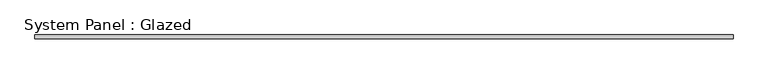
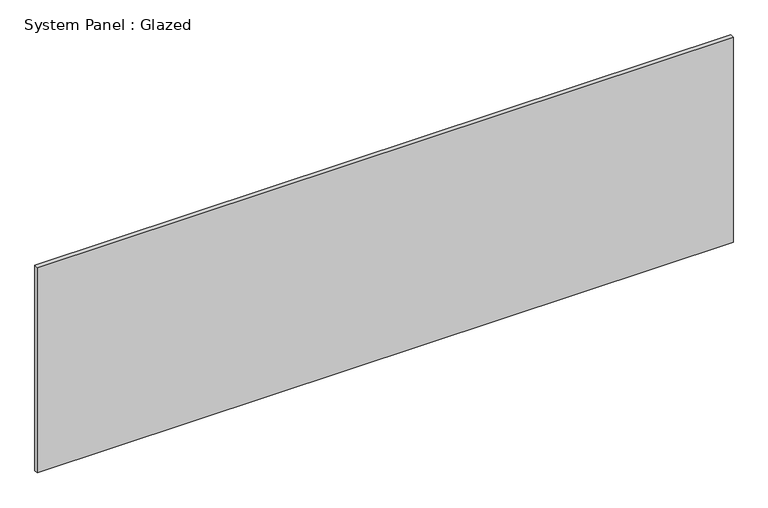
"""IFC4 building model written with IfcOpenShell, lengths in millimetres: plate geometry, System Panel : Glazed."""

from ifc_helpers import new_model, si_unit, origin, origin_with_axes, place, context, project, spatial, polyline, outline, extrude, source, transform, mapped, element, save


def system_panel_glazed_dcdbdfd1(model_context):
    return source(origin(), model_context, "Body", "SweptSolid", [
        extrude(outline(polyline([(2343.15, 19.05), (-2343.15, 19.05), (-2343.15, 44.45), (2343.15, 44.45), (2343.15, 19.05)])), origin_with_axes(), (0.0, 0.0, 1.0), 1460.5),
    ])


if __name__ == "__main__":
    model = new_model("IFC4")
    model_context = context("Model", 3, world=origin())
    ifc_project = project(units=[si_unit("LENGTHUNIT", "METRE", prefix="MILLI")], contexts=[model_context])
    site = spatial("IfcSite", under=ifc_project)
    building = spatial("IfcBuilding", under=site)
    placement = place(None, origin())
    system_panel_glazed_shape = system_panel_glazed_dcdbdfd1(model_context)
    element("IfcPlate", 1, ObjectType="System Panel : Glazed", at=placement, inside=building, context=model_context, shape_type="MappedRepresentation", body=[
        mapped(system_panel_glazed_shape, transform((0.0, 0.0, 0.0), x_axis=(1.0, 0.0, 0.0), y_axis=(0.0, 1.0, 0.0), z_axis=(0.0, 0.0, 1.0))),
    ])
    save(model, "model.ifc")

# Revit data of these elements
# Type "System Panel : Glazed"
#   Construction Type Id = "GSP4R"
#   Analytic Construction = "1/8 in Pilkington single glazing"
#   Visual Light Transmittance = 0.9
#   Solar Heat Gain Coefficient = 0.86
#   Heat Transfer Coefficient (U) = 1.18115 BTU/(h·ft²·°F)
# Element 1 (IfcPlate, "System Panel : Glazed")
#   Materials on its faces: "Glass"
# Materials
#   "Glass": class "Glass", colour RGB 0 128 192, transparency 0.75, Description = "Soda Lime Glass", Cost = 0
